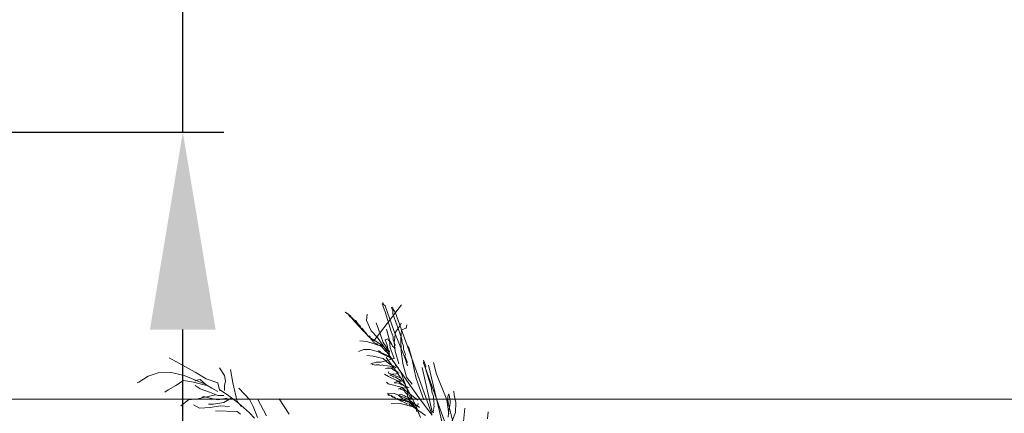
# Model space of a CAD drawing. Units: millimetres. Extents: x 595116 to 630915, y 909473 to 920225.
# Tile 64 of 134: x 629589 to 629619, y 919302 to 919314. Entities that reach past the tile are written whole.
import ezdxf

# ---------------------------------------------------------------- set-up
doc = ezdxf.new("R2010")
doc.units = ezdxf.units.MM
doc.layers.add('Dimension', color=3, linetype='Continuous', lineweight=18)
doc.layers.add('L-PLNT', color=85, linetype='Continuous', lineweight=13)
doc.styles.get("Standard").update_dxf_attribs({"font": 'arial.ttf'})
doc.dimstyles.new('ISO-25', dxfattribs={"dimtxt": 9, "dimasz": 6, "dimexe": 1.25, "dimexo": 0.625, "dimtad": 1, "dimlunit": 4, "dimtxsty": 'Standard', "dimcen": 2.5, "dimadec": 0, "dimazin": 0, "dimtfac": 1, "dimtmove": 0, "dimatfit": 3, "dimfxl": 1, "dimarcsym": 0})

# ---------------------------------------------------------------- blocks, each defined once
blk = doc.blocks.new('A$C4FB75ABC')
for p, q in [((2.2354, 4.7176), (2.2283, 4.715)), ((2.2283, 4.715), (2.2515, 4.6504)), ((2.238, 4.7104), (2.2329, 4.7248)), ((2.2329, 4.7248), (2.2354, 4.7176)), ((2.2504, 4.6987), (2.238, 4.7104)), ((1.9382, 4.6431), (1.9285, 4.6477)), ((1.9285, 4.6477), (1.9408, 4.6359)), ((1.9506, 4.6313), (1.9382, 4.6431)), ((1.9408, 4.6359), (1.9506, 4.6313)), ((1.9603, 4.6267), (1.9506, 4.6313)), ((1.9506, 4.6313), (1.9655, 4.6124)), ((2.0989, 4.5793), (2.1049, 4.6301)), ((2.1583, 4.4143), (2.3852, 4.7066)), ((2.3227, 4.4977), (2.2504, 4.6987)), ((2.2515, 4.6504), (2.3011, 4.49)), ((2.3109, 4.688), (2.3037, 4.6854)), ((2.3037, 4.6854), (2.314, 4.6567)), ((2.3186, 4.6665), (2.3109, 4.688)), ((2.314, 4.6567), (2.3146, 4.6326)), ((2.3146, 4.6326), (2.3843, 4.4389)), ((2.3336, 4.6475), (2.3186, 4.6665)), ((2.6279, 3.8295), (2.3336, 4.6475)), ((1.9726, 4.6149), (1.9603, 4.6267)), ((1.9655, 4.6124), (1.9778, 4.6006)), ((1.9752, 4.6078), (1.9726, 4.6149)), ((1.985, 4.6032), (1.9752, 4.6078)), ((1.9778, 4.6006), (2.0051, 4.5699)), ((1.9876, 4.596), (1.985, 4.6032)), ((1.9973, 4.5914), (1.9876, 4.596)), ((1.9999, 4.5842), (1.9973, 4.5914)), ((2.0097, 4.5796), (1.9999, 4.5842)), ((2.1238, 4.4424), (2.0025, 4.577)), ((2.0051, 4.5699), (2.0174, 4.5581)), ((2.0194, 4.575), (2.0097, 4.5796)), ((2.0174, 4.5581), (2.0323, 4.5391)), ((2.0246, 4.5607), (2.0194, 4.575)), ((2.0395, 4.5417), (2.0246, 4.5607)), ((2.137, 4.4958), (2.0989, 4.5793)), ((2.197, 4.5092), (2.1789, 4.5595)), ((2.3723, 4.5399), (2.3815, 4.5594)), ((2.0323, 4.5391), (2.0447, 4.5274)), ((2.0493, 4.5371), (2.0395, 4.5417)), ((2.0447, 4.5274), (2.0719, 4.4967)), ((2.057, 4.5156), (2.0493, 4.5371)), ((2.0642, 4.5182), (2.057, 4.5156)), ((2.0668, 4.511), (2.0642, 4.5182)), ((2.0791, 4.4992), (2.0668, 4.511)), ((2.0719, 4.4967), (2.0966, 4.4731)), ((2.0817, 4.4921), (2.0791, 4.4992)), ((2.094, 4.4803), (2.0817, 4.4921)), ((2.1115, 4.4542), (2.094, 4.4803)), ((2.0966, 4.4731), (2.1115, 4.4542)), ((2.189, 4.4415), (2.137, 4.4958)), ((2.2357, 4.4016), (2.197, 4.5092)), ((2.2859, 4.4197), (2.2621, 4.5084)), ((2.3011, 4.49), (2.3166, 4.4469)), ((2.4125, 4.2707), (2.3227, 4.4977)), ((2.325, 4.4013), (2.335, 4.486)), ((2.335, 4.486), (2.3723, 4.5399)), ((2.3797, 4.4291), (2.3852, 4.504)), ((2.3852, 4.504), (2.4211, 4.5169)), ((2.4211, 4.5169), (2.4277, 4.5436)), ((2.1029, 4.4105), (2.0449, 4.414)), ((2.222, 4.3723), (2.1029, 4.4105)), ((2.1238, 4.4424), (2.1115, 4.4542)), ((2.1115, 4.4542), (2.1284, 4.4522)), ((2.1336, 4.4378), (2.1238, 4.4424)), ((2.185, 4.4077), (2.1238, 4.4424)), ((2.1284, 4.4522), (2.1336, 4.4378)), ((2.1388, 4.4235), (2.1336, 4.4378)), ((2.1336, 4.4378), (2.1434, 4.4332)), ((2.1485, 4.4189), (2.1388, 4.4235)), ((2.1434, 4.4332), (2.1485, 4.4189)), ((2.1485, 4.4189), (2.1557, 4.4214)), ((2.1537, 4.4045), (2.1485, 4.4189)), ((2.1609, 4.4071), (2.1537, 4.4045)), ((2.1557, 4.4214), (2.1583, 4.4143)), ((2.1634, 4.3999), (2.1609, 4.4071)), ((2.1829, 4.3907), (2.1634, 4.3999)), ((2.1953, 4.379), (2.1829, 4.3907)), ((2.2389, 4.3703), (2.185, 4.4077)), ((2.2564, 4.3442), (2.189, 4.4415)), ((2.2882, 4.3232), (2.2357, 4.4016)), ((2.2736, 4.4314), (2.2521, 4.4237)), ((2.2521, 4.4237), (2.2676, 4.3807)), ((2.2788, 4.4171), (2.2736, 4.4314)), ((2.2885, 4.4125), (2.2788, 4.4171)), ((2.2922, 4.3571), (2.2859, 4.4197)), ((2.306, 4.3864), (2.2885, 4.4125)), ((2.3166, 4.4469), (2.3172, 4.4228)), ((2.3172, 4.4228), (2.3327, 4.3798)), ((2.3338, 4.3316), (2.325, 4.4013)), ((2.382, 4.3327), (2.3797, 4.4291)), ((2.3843, 4.4389), (2.3901, 4.4004)), ((2.3901, 4.4004), (2.4004, 4.3717)), ((2.0779, 4.3448), (2.0349, 4.3293)), ((2.1261, 4.346), (2.0779, 4.3448)), ((2.1893, 4.3282), (2.1261, 4.346)), ((2.277, 4.2868), (2.1893, 4.3282)), ((2.1938, 4.3379), (2.1964, 4.3307)), ((2.2122, 4.3769), (2.1953, 4.379)), ((2.1964, 4.3307), (2.2036, 4.3333)), ((2.2036, 4.3333), (2.2062, 4.3261)), ((2.2062, 4.3261), (2.2134, 4.3287)), ((2.2245, 4.3652), (2.2122, 4.3769)), ((2.2134, 4.3287), (2.2159, 4.3215)), ((2.2159, 4.3215), (2.2354, 4.3124)), ((2.2518, 4.3344), (2.2245, 4.3652)), ((2.2354, 4.3124), (2.2452, 4.3078)), ((2.2785, 4.3278), (2.2389, 4.3703)), ((2.2641, 4.3227), (2.2518, 4.3344)), ((2.2538, 4.3417), (2.3557, 4.1924)), ((2.2765, 4.3109), (2.2641, 4.3227)), ((2.2676, 4.3807), (2.2759, 4.335)), ((2.2759, 4.335), (2.2862, 4.3063)), ((2.2791, 4.3037), (2.2765, 4.3109)), ((2.3232, 4.271), (2.2922, 4.3571)), ((2.3112, 4.372), (2.306, 4.3864)), ((2.3235, 4.3603), (2.3112, 4.372)), ((2.3261, 4.3531), (2.3235, 4.3603)), ((2.3333, 4.3557), (2.3261, 4.3531)), ((2.3327, 4.3798), (2.3281, 4.37)), ((2.3281, 4.37), (2.3333, 4.3557)), ((2.3628, 4.2285), (2.3338, 4.3316)), ((2.3941, 4.2317), (2.382, 4.3327)), ((2.4004, 4.3717), (2.401, 4.3476)), ((2.401, 4.3476), (2.4165, 4.3046)), ((2.4678, 4.2744), (2.4414, 4.3703)), ((0.4999, 4.2779), (0.7111, 4.1621)), ((2.154, 4.2911), (2.1032, 4.2972)), ((2.1362, 4.228), (2.1792, 4.2435)), ((2.234, 4.2713), (2.154, 4.2911)), ((2.1792, 4.2435), (2.1961, 4.2415)), ((2.1961, 4.2415), (2.2202, 4.242)), ((2.2202, 4.242), (2.3304, 4.2736)), ((2.2808, 4.2314), (2.234, 4.2713)), ((2.2452, 4.3078), (2.255, 4.3032)), ((2.255, 4.3032), (2.2745, 4.294)), ((2.3407, 4.1707), (2.2593, 4.2788)), ((2.2745, 4.294), (2.2868, 4.2822)), ((2.2862, 4.3063), (2.2791, 4.3037)), ((2.3419, 4.1967), (2.2808, 4.2314)), ((2.2868, 4.2822), (2.2991, 4.2704)), ((2.2991, 4.2704), (2.3089, 4.2658)), ((2.3089, 4.2658), (2.3166, 4.2443)), ((2.3166, 4.2443), (2.3264, 4.2397)), ((2.3264, 4.2397), (2.3341, 4.2182)), ((2.4257, 4.1214), (2.3941, 4.2317)), ((2.4165, 4.3046), (2.4119, 4.2948)), ((2.4119, 4.2948), (2.43, 4.2446)), ((2.4331, 4.2133), (2.4125, 4.2707)), ((2.43, 4.2446), (2.4279, 4.2276)), ((2.4896, 4.1688), (2.4678, 4.2744)), ((2.5803, 4.2095), (2.5622, 4.2597)), ((2.5622, 4.2597), (2.5648, 4.2526)), ((2.5648, 4.2526), (2.5628, 4.2356)), ((2.5628, 4.2356), (2.5757, 4.1997)), ((2.6686, 4.144), (2.6423, 4.2399)), ((0.4114, 4.1553), (0.3296, 4.1281)), ((0.5068, 4.1621), (0.4114, 4.1553)), ((0.6226, 4.1349), (0.5068, 4.1621)), ((0.7111, 4.1621), (0.7997, 4.1076)), ((0.9087, 4.1962), (0.9496, 4.1349)), ((0.9973, 4.1826), (1.0177, 4.0736)), ((2.1434, 4.2306), (2.1362, 4.228)), ((2.1459, 4.2234), (2.1434, 4.2306)), ((2.1629, 4.2214), (2.1459, 4.2234)), ((2.1726, 4.2168), (2.1629, 4.2214)), ((2.1798, 4.2194), (2.1726, 4.2168)), ((2.2039, 4.22), (2.1798, 4.2194)), ((2.2136, 4.2154), (2.2039, 4.22)), ((2.228, 4.2205), (2.2136, 4.2154)), ((2.2377, 4.2159), (2.228, 4.2205)), ((2.2716, 4.2119), (2.2377, 4.2159)), ((2.2552, 4.1898), (2.2768, 4.1975)), ((2.2696, 4.195), (2.2552, 4.1898)), ((2.2793, 4.1904), (2.2696, 4.195)), ((2.2885, 4.2099), (2.2716, 4.2119)), ((2.2753, 4.1565), (2.2799, 4.1663)), ((2.38, 4.1131), (2.2753, 4.1565)), ((2.2768, 4.1975), (2.2865, 4.1929)), ((2.2865, 4.1929), (2.2793, 4.1904)), ((2.2865, 4.1929), (2.3106, 4.1935)), ((2.3034, 4.1909), (2.2865, 4.1929)), ((2.308, 4.2007), (2.2885, 4.2099)), ((2.3353, 4.17), (2.3034, 4.1909)), ((2.3178, 4.1961), (2.308, 4.2007)), ((2.3106, 4.1935), (2.325, 4.1987)), ((2.325, 4.1987), (2.3178, 4.1961)), ((2.3341, 4.2182), (2.3465, 4.2064)), ((2.345, 4.1654), (2.3353, 4.17)), ((2.3359, 4.1459), (2.3645, 4.1562)), ((2.4072, 4.0691), (2.3407, 4.1707)), ((2.3548, 4.1608), (2.345, 4.1654)), ((2.3465, 4.2064), (2.3588, 4.1946)), ((2.3574, 4.1536), (2.3548, 4.1608)), ((2.3557, 4.1924), (2.443, 4.0685)), ((2.3645, 4.1562), (2.3574, 4.1536)), ((2.3588, 4.1946), (2.364, 4.1803)), ((2.364, 4.1803), (2.3789, 4.1614)), ((2.3789, 4.1614), (2.4357, 4.0035)), ((2.4279, 4.2276), (2.4331, 4.2133)), ((2.5031, 4.1088), (2.4896, 4.1688)), ((2.6325, 3.8393), (2.5516, 4.1992)), ((2.5757, 4.1997), (2.6279, 4.0321)), ((2.5783, 4.1926), (2.5803, 4.2095)), ((2.8029, 3.5683), (2.5783, 4.1926)), ((2.7169, 3.7399), (2.6018, 4.2172)), ((0.2547, 4.0804), (0.241, 4.0736)), ((0.3296, 4.1281), (0.2547, 4.0804)), ((0.6158, 4.094), (0.5544, 4.0532)), ((0.6975, 4.0804), (0.6158, 4.094)), ((0.7861, 4.0668), (0.6226, 4.1349)), ((0.8065, 4.0532), (0.6975, 4.0804)), ((0.752, 4.1008), (0.7111, 4.094)), ((0.7111, 4.094), (0.7111, 4.0872)), ((0.7997, 4.06), (0.752, 4.1008)), ((0.7997, 4.1076), (0.8951, 4.0736)), ((0.8951, 4.0736), (0.9087, 4.0191)), ((0.9496, 4.1349), (0.9564, 4.0872)), ((0.9564, 4.0872), (0.9496, 4.0532)), ((1.0177, 4.0736), (1.0518, 3.9238)), ((2.2785, 4.1252), (2.2466, 4.1462)), ((2.275, 4.0672), (2.2627, 4.079)), ((2.3468, 4.0931), (2.2785, 4.1252)), ((2.2902, 4.1376), (2.3189, 4.1479)), ((2.3, 4.133), (2.2902, 4.1376)), ((2.3098, 4.1284), (2.3, 4.133)), ((2.3195, 4.1238), (2.3098, 4.1284)), ((2.3189, 4.1479), (2.3359, 4.1459)), ((2.3364, 4.1218), (2.3195, 4.1238)), ((2.3278, 4.0781), (2.3565, 4.0885)), ((2.3304, 4.071), (2.3278, 4.0781)), ((2.3448, 4.0761), (2.3304, 4.071)), ((2.3585, 4.1054), (2.3364, 4.1218)), ((2.3714, 4.0695), (2.3448, 4.0761)), ((2.413, 4.044), (2.3468, 4.0931)), ((2.3565, 4.0885), (2.3806, 4.089)), ((2.3683, 4.1008), (2.3585, 4.1054)), ((2.3806, 4.089), (2.3683, 4.1008)), ((2.3806, 4.089), (2.395, 4.0942)), ((2.395, 4.0942), (2.3806, 4.089)), ((2.4704, 4.0646), (2.4257, 4.1214)), ((2.5651, 3.9366), (2.5031, 4.1088)), ((2.7507, 3.9385), (2.6686, 4.144)), ((0.4931, 4.0191), (0.4659, 3.9987)), ((0.5544, 4.0532), (0.4931, 4.0191)), ((0.7111, 4.0532), (0.752, 4.0259)), ((0.752, 4.0259), (0.827, 3.9987)), ((0.8474, 4.0327), (0.7997, 4.06)), ((0.827, 3.9987), (0.8951, 3.9715)), ((0.8951, 4.0055), (0.8474, 4.0327)), ((0.9842, 3.9699), (0.9085, 4.0207)), ((0.9087, 4.0191), (0.9087, 4.0123)), ((0.9496, 4.0532), (0.9496, 4.0123)), ((1.0654, 4.0327), (1.154, 3.9374)), ((2.3275, 3.9889), (2.2696, 3.9923)), ((2.3818, 4.0408), (2.275, 4.0672)), ((2.3557, 4.0233), (2.3915, 4.0362)), ((2.37, 4.0285), (2.3557, 4.0233)), ((2.3798, 4.0239), (2.37, 4.0285)), ((2.3838, 4.0577), (2.3714, 4.0695)), ((2.3993, 4.0147), (2.3798, 4.0239)), ((2.5169, 3.9354), (2.3818, 4.0408)), ((2.3909, 4.0603), (2.3838, 4.0577)), ((2.413, 4.044), (2.3909, 4.0603)), ((2.3915, 4.0362), (2.4013, 4.0316)), ((2.409, 4.0101), (2.3993, 4.0147)), ((2.4013, 4.0316), (2.4084, 4.0342)), ((2.4608, 3.9732), (2.4072, 4.0691)), ((2.4084, 4.0342), (2.4325, 4.0348)), ((2.4142, 3.9957), (2.409, 4.0101)), ((2.43, 4.0419), (2.413, 4.044)), ((2.4363, 3.9794), (2.4142, 3.9957)), ((2.4325, 4.0348), (2.43, 4.0419)), ((2.4357, 4.0035), (2.4311, 3.9937)), ((2.4311, 3.9937), (2.4337, 3.9866)), ((2.4325, 4.0348), (2.4469, 4.0399)), ((2.4469, 4.0399), (2.4325, 4.0348)), ((2.443, 4.0685), (2.5171, 3.9664)), ((2.6279, 4.0321), (2.6311, 4.0008)), ((2.6311, 4.0008), (2.644, 3.965)), ((2.8101, 3.9761), (2.8069, 4.0074)), ((0.6566, 3.9374), (0.5953, 3.8897)), ((0.7316, 3.9442), (0.6566, 3.9374)), ((0.8746, 3.9783), (0.7316, 3.9442)), ((0.7793, 3.9647), (0.7656, 3.9578)), ((0.8338, 3.951), (0.7793, 3.9647)), ((0.8951, 3.9374), (0.8338, 3.951)), ((0.9428, 3.917), (0.861, 3.9034)), ((0.8951, 3.9715), (0.9428, 3.9715)), ((0.97, 3.951), (0.8951, 3.9374)), ((1.0041, 3.951), (0.9428, 3.917)), ((1.0487, 3.9217), (0.9842, 3.9699)), ((1.1035, 3.8758), (1.0487, 3.9217)), ((1.0518, 3.9238), (1.0858, 3.8829)), ((1.154, 3.9374), (1.1812, 3.8829)), ((1.2153, 3.9442), (1.2902, 3.808)), ((1.3924, 3.9442), (1.4742, 3.8217)), ((2.2748, 3.978), (2.2722, 3.9852)), ((2.2722, 3.9852), (2.2748, 3.978)), ((2.2748, 3.978), (2.2819, 3.9806)), ((2.2845, 3.9734), (2.2748, 3.978)), ((2.2819, 3.9806), (2.2917, 3.976)), ((2.2917, 3.976), (2.2845, 3.9734)), ((2.3014, 3.9714), (2.2917, 3.976)), ((2.2917, 3.976), (2.3014, 3.9714)), ((2.304, 3.9642), (2.3014, 3.9714)), ((2.3014, 3.9714), (2.3138, 3.9596)), ((2.3112, 3.9668), (2.304, 3.9642)), ((2.3138, 3.9596), (2.3112, 3.9668)), ((2.3209, 3.9622), (2.3138, 3.9596)), ((2.3138, 3.9596), (2.3235, 3.955)), ((2.3307, 3.9576), (2.3209, 3.9622)), ((2.3235, 3.955), (2.3333, 3.9504)), ((2.4323, 3.9455), (2.3275, 3.9889)), ((2.3333, 3.9504), (2.3307, 3.9576)), ((2.343, 3.9458), (2.3333, 3.9504)), ((2.3333, 3.9504), (2.343, 3.9458)), ((2.3502, 3.9484), (2.343, 3.9458)), ((2.343, 3.9458), (2.3697, 3.9392)), ((2.3528, 3.9412), (2.3502, 3.9484)), ((2.3723, 3.932), (2.3528, 3.9412)), ((2.3568, 3.9751), (2.3783, 3.9828)), ((2.3691, 3.9633), (2.3568, 3.9751)), ((2.3789, 3.9587), (2.3691, 3.9633)), ((2.3697, 3.9392), (2.3821, 3.9274)), ((2.3866, 3.9372), (2.3723, 3.932)), ((2.3783, 3.9828), (2.3881, 3.9782)), ((2.3912, 3.947), (2.3789, 3.9587)), ((2.3821, 3.9274), (2.3918, 3.9228)), ((2.3892, 3.93), (2.3866, 3.9372)), ((2.3881, 3.9782), (2.4076, 3.9691)), ((2.3964, 3.9326), (2.3892, 3.93)), ((2.401, 3.9424), (2.3912, 3.947)), ((2.3918, 3.9228), (2.4113, 3.9137)), ((2.4133, 3.9306), (2.3964, 3.9326)), ((2.44, 3.924), (2.401, 3.9424)), ((2.4076, 3.9691), (2.4173, 3.9645)), ((2.4113, 3.9137), (2.4211, 3.9091)), ((2.4159, 3.9234), (2.4133, 3.9306)), ((2.4231, 3.926), (2.4159, 3.9234)), ((2.4173, 3.9645), (2.4368, 3.9553)), ((2.4328, 3.9214), (2.4231, 3.926)), ((2.4337, 3.9866), (2.4291, 3.9768)), ((2.4291, 3.9768), (2.442, 3.9409)), ((2.5304, 3.8755), (2.4323, 3.9455)), ((2.4498, 3.9194), (2.4328, 3.9214)), ((2.446, 3.9748), (2.4363, 3.9794)), ((2.4368, 3.9553), (2.4466, 3.9507)), ((2.4523, 3.9122), (2.44, 3.924)), ((2.442, 3.9409), (2.4569, 3.922)), ((2.4512, 3.9604), (2.446, 3.9748)), ((2.4466, 3.9507), (2.4635, 3.9487)), ((2.4595, 3.9148), (2.4498, 3.9194)), ((2.4609, 3.9558), (2.4512, 3.9604)), ((2.477, 3.8887), (2.4523, 3.9122)), ((2.4569, 3.922), (2.4667, 3.9174)), ((2.4621, 3.9076), (2.4595, 3.9148)), ((2.5035, 3.8821), (2.4608, 3.9732)), ((2.4635, 3.9487), (2.4609, 3.9558)), ((2.4667, 3.9174), (2.4693, 3.9102)), ((2.5171, 3.9664), (2.5794, 3.8826)), ((2.644, 3.965), (2.6451, 3.9167)), ((2.6451, 3.9167), (2.6477, 3.9096)), ((2.7679, 3.8231), (2.7507, 3.9385)), ((2.7619, 3.975), (2.7599, 3.958)), ((2.7599, 3.958), (2.7605, 3.9339)), ((2.7605, 3.9339), (2.7636, 3.9026)), ((2.7665, 3.9847), (2.7619, 3.975)), ((2.7742, 3.9632), (2.7665, 3.9847)), ((2.7748, 3.9391), (2.7742, 3.9632)), ((2.7774, 3.9319), (2.7748, 3.9391)), ((2.778, 3.9078), (2.7774, 3.9319)), ((2.8236, 3.9161), (2.8101, 3.9761)), ((2.8207, 3.834), (2.8236, 3.9161)), ((0.7452, 3.8693), (0.6975, 3.8966)), ((0.8338, 3.8761), (0.7452, 3.8693)), ((0.861, 3.9034), (0.8201, 3.9034)), ((0.9155, 3.8897), (0.8338, 3.8761)), ((0.8746, 3.8489), (1.0518, 3.8421)), ((0.9905, 3.8829), (0.9155, 3.8897)), ((1.0518, 3.8421), (1.079, 3.8217)), ((1.1506, 3.8319), (1.1035, 3.8758)), ((1.1917, 3.7897), (1.1506, 3.8319)), ((1.1812, 3.8829), (1.2017, 3.8285)), ((2.3729, 3.9079), (2.3006, 3.9062)), ((2.4796, 3.8815), (2.3729, 3.9079)), ((2.4211, 3.9091), (2.4237, 3.9019)), ((2.4237, 3.9019), (2.4308, 3.9045)), ((2.4308, 3.9045), (2.4478, 3.9025)), ((2.4478, 3.9025), (2.4503, 3.8953)), ((2.4503, 3.8953), (2.4698, 3.8861)), ((2.4718, 3.903), (2.4621, 3.9076)), ((2.4693, 3.9102), (2.479, 3.9056)), ((2.4698, 3.8861), (2.4796, 3.8815)), ((2.4842, 3.8913), (2.4718, 3.903)), ((2.4868, 3.8841), (2.477, 3.8887)), ((2.479, 3.9056), (2.4868, 3.8841)), ((2.4796, 3.8815), (2.4868, 3.8841)), ((2.5777, 3.8114), (2.4796, 3.8815)), ((2.4914, 3.8938), (2.4842, 3.8913)), ((2.4868, 3.8841), (2.4893, 3.8769)), ((2.4919, 3.8697), (2.4868, 3.8841)), ((2.4868, 3.8841), (2.4991, 3.8723)), ((2.4893, 3.8769), (2.4991, 3.8723)), ((2.5011, 3.8892), (2.4914, 3.8938)), ((2.5063, 3.8749), (2.4919, 3.8697)), ((2.4991, 3.8723), (2.5063, 3.8749)), ((2.4991, 3.8723), (2.5094, 3.8436)), ((2.5155, 3.8944), (2.5011, 3.8892)), ((2.5372, 3.7949), (2.5035, 3.8821)), ((2.5094, 3.8436), (2.5166, 3.8462)), ((2.52, 3.9042), (2.5155, 3.8944)), ((2.5166, 3.8462), (2.5244, 3.8247)), ((2.5175, 3.9113), (2.52, 3.9042)), ((2.5794, 3.8826), (2.6314, 3.8136)), ((2.6423, 3.8347), (2.6279, 3.8295)), ((2.6443, 3.8516), (2.6397, 3.8418)), ((2.6397, 3.8418), (2.6423, 3.8347)), ((2.6463, 3.8685), (2.6417, 3.8588)), ((2.6417, 3.8588), (2.6443, 3.8516)), ((2.6477, 3.9096), (2.6457, 3.8926)), ((2.6457, 3.8926), (2.6483, 3.8855)), ((2.6483, 3.8855), (2.6463, 3.8685)), ((2.7636, 3.9026), (2.8247, 3.6653)), ((2.7653, 3.8303), (2.7673, 3.8473)), ((2.7673, 3.8473), (2.7739, 3.8739)), ((2.7739, 3.8739), (2.778, 3.9078)), ((2.7957, 3.7683), (2.8207, 3.834)), ((2.8876, 3.7608), (2.897, 3.8696)), ((3.0823, 3.7823), (3.0858, 3.8403)), ((1.2017, 3.8285), (1.2153, 3.7944)), ((2.7613, 3.7965), (2.7653, 3.8303))]:
    blk.add_line(p, q)
blk = doc.blocks.new('*D210')
at = {"layer": 'Defpoints', "color": 0, "transparency": 16777216}
for p in [(629586.227, 919310.123), (629593.946, 919310.123), (629586.227, 919258.662)]:
    blk.add_point(p, dxfattribs=at)
at = {"layer": 'Dimension', "color": 0, "lineweight": -2, "transparency": 16777216}
for p, q in [((629593.946, 919310.123), (629593.946, 919449.69)), ((629586.852, 919310.123), (629595.196, 919310.123)), ((629593.946, 919264.662), (629593.946, 919304.123)), ((629586.852, 919258.662), (629595.196, 919258.662))]:
    blk.add_line(p, q, dxfattribs=at)
at = {"layer": 'Dimension', "color": 0, "transparency": 16777216}
for points in [[(629592.946, 919304.123), (629594.946, 919304.123), (629593.946, 919310.123)], [(629592.946, 919264.662), (629594.946, 919264.662), (629593.946, 919258.662)]]:
    blk.add_solid(points, dxfattribs=at)
at = {"layer": 'Dimension', "color": 0, "transparency": 16777216, "insert": (629588.662, 919382.907), "char_height": 9, "attachment_point": 5, "rotation": 90}
blk.add_mtext('CANOPY 4\'-3 1/2" TYP.', dxfattribs=at)
blk = doc.blocks.new('*D216')
at = {"layer": 'Defpoints', "color": 0, "transparency": 16777216}
for p in [(629743.541, 919411.928), (629505.041, 919411.828), (629743.541, 918832.378)]:
    blk.add_point(p, dxfattribs=at)
at = {"layer": 'Dimension', "color": 0, "lineweight": -2, "transparency": 16777216}
for p, q in [((629505.041, 919411.203), (629505.041, 918831.128)), ((629743.541, 919411.303), (629743.541, 918831.128)), ((629511.041, 918832.378), (629737.541, 918832.378))]:
    blk.add_line(p, q, dxfattribs=at)
at = {"layer": 'Dimension', "color": 0, "transparency": 16777216}
for points in [[(629511.041, 918833.378), (629511.041, 918831.378), (629505.041, 918832.378)], [(629737.541, 918833.378), (629737.541, 918831.378), (629743.541, 918832.378)]]:
    blk.add_solid(points, dxfattribs=at)
at = {"layer": 'Dimension', "color": 0, "transparency": 16777216, "insert": (629624.291, 918837.656), "char_height": 9, "attachment_point": 5}
blk.add_mtext('19\'-10 1/2"', dxfattribs=at)
blk = doc.blocks.new('*D220')
at = {"layer": 'Defpoints', "color": 0, "transparency": 16777216}
for p in [(629824.951, 920160.756), (629511.274, 919302.009), (629824.951, 919302.009)]:
    blk.add_point(p, dxfattribs=at)
at = {"layer": 'Dimension', "color": 0, "lineweight": -2, "transparency": 16777216}
for p, q in [((629511.274, 919302.634), (629511.274, 920162.006)), ((629824.951, 919302.634), (629824.951, 920162.006)), ((629517.274, 920160.756), (629818.951, 920160.756))]:
    blk.add_line(p, q, dxfattribs=at)
at = {"layer": 'Dimension', "color": 0, "transparency": 16777216}
for points in [[(629517.274, 920161.756), (629517.274, 920159.756), (629511.274, 920160.756)], [(629818.951, 920161.756), (629818.951, 920159.756), (629824.951, 920160.756)]]:
    blk.add_solid(points, dxfattribs=at)
at = {"layer": 'Dimension', "color": 0, "transparency": 16777216, "insert": (629668.113, 920166.035), "char_height": 9, "attachment_point": 5}
blk.add_mtext('26\'-1 1/2"', dxfattribs=at)

msp = doc.modelspace()

# ---------------------------------------------------------------- linework, layer by layer
at = {"layer": 'L-PLNT'}
msp.add_line((629824.951, 919302.009), (629511.274, 919302.009), dxfattribs=at)

# ---------------------------------------------------------------- block references
at = {"layer": 'L-PLNT', "xscale": 3.753413438031968, "yscale": 3.753413438031968, "zscale": 3.753413438031968}
msp.add_blockref('A$C4FB75ABC', (629591.653, 919287.212), dxfattribs=at)

# ---------------------------------------------------------------- dimensions: what is measured, and where the dimension line sits
at = {"layer": 'Dimension'}
for base, p1, p2, picture, middle in [((629824.951, 920160.756), (629511.274, 919302.009), (629824.951, 919302.009), '*D220', (629668.113, 920166.035)), ((629743.541, 918832.378), (629505.041, 919411.828), (629743.541, 919411.928), '*D216', (629624.291, 918837.656))]:
    dim = msp.add_linear_dim(base=base, p1=p1, p2=p2, dimstyle='ISO-25', override={"dimdec": 1, "dimlfac": 1, "dimrnd": 0, "dimzin": 1, "dimdsep": 46, "dimlunit": 4, "dimfrac": 2}, dxfattribs=at)
    dim.commit()
    dim.dimension.update_dxf_attribs({"geometry": picture, "text_midpoint": middle})
dim = msp.add_linear_dim(base=(629593.946, 919310.123), p1=(629586.227, 919258.662), p2=(629586.227, 919310.123), angle=90, text='CANOPY <> TYP.', dimstyle='ISO-25', override={"dimdec": 1, "dimlfac": 1, "dimrnd": 0, "dimzin": 1, "dimdsep": 46, "dimlunit": 4, "dimfrac": 2}, dxfattribs=at)
dim.commit()
dim.dimension.update_dxf_attribs({"geometry": '*D210', "text_midpoint": (629588.662, 919382.907)})

doc.saveas('drawing.dxf')
